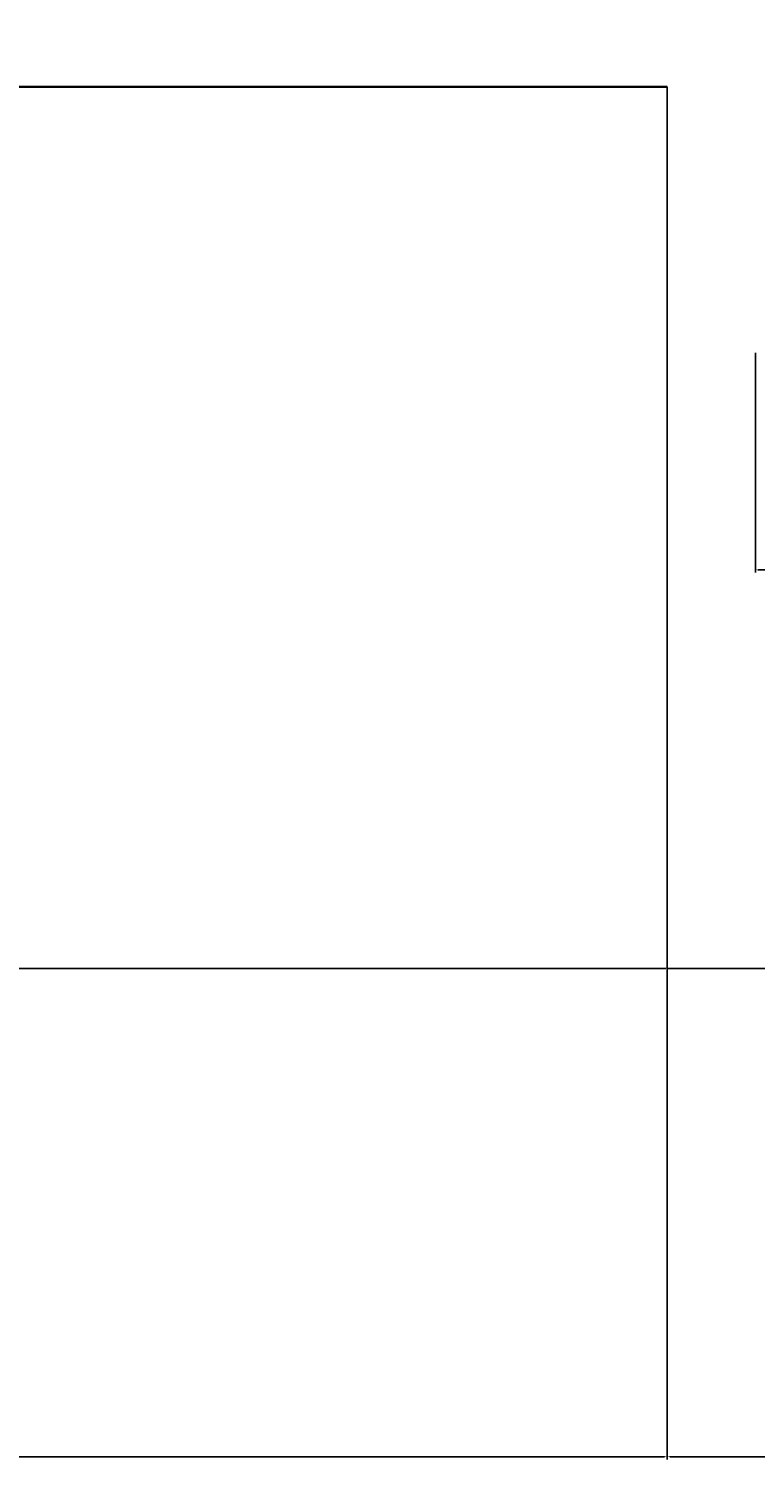
# Model space of a CAD drawing. Units: inches. Extents: x 4159 to 4826, y 299 to 1026.
# Tile 7 of 37: x 4404 to 4453, y 299 to 396. Entities that reach past the tile are written whole.
import ezdxf

# ---------------------------------------------------------------- set-up
doc = ezdxf.new("R2010")
doc.units = ezdxf.units.IN
for name, color, linetype, lineweight in [('A-ANNO-DIMS', 2, 'Continuous', 18), ('A-FLOR-STRS', 3, 'Continuous', 25), ('A-WALL', 7, 'Continuous', 35)]:
    doc.layers.add(name, color=color, linetype=linetype, lineweight=lineweight)
doc.styles.get("Standard").update_dxf_attribs({"font": 'arial.ttf'})
doc.dimstyles.get("Standard").update_dxf_attribs({"dimtxt": 0.18, "dimasz": 0.18, "dimexe": 0.18, "dimexo": 0.0625, "dimgap": 0.09, "dimtad": 0, "dimtih": 1, "dimtoh": 1, "dimdec": 4, "dimzin": 0, "dimdsep": 46, "dimtxsty": 'Standard', "dimcen": 0.09, "dimadec": 0, "dimazin": 0, "dimtfac": 1, "dimtdec": 4, "dimtofl": 0, "dimtmove": 0, "dimatfit": 3, "dimfxl": 1, "dimtolj": 1, "dimtzin": 0, "dimarcsym": 0})

# ---------------------------------------------------------------- blocks, each defined once
blk = doc.blocks.new('*D42')
at = {"layer": 'A-ANNO-DIMS', "color": 0, "lineweight": -2, "transparency": 16777216}
for p, q in [((4453.31, 374.133), (4453.31, 359.165)), ((4495.889, 374.133), (4495.889, 359.165)), ((4453.49, 359.345), (4474.068, 359.345)), ((4495.709, 359.345), (4475.131, 359.345))]:
    blk.add_line(p, q, dxfattribs=at)
at = {"layer": 'A-ANNO-DIMS', "color": 0, "transparency": 16777216}
for points in [[(4453.49, 359.375), (4453.49, 359.315), (4453.31, 359.345)], [(4495.709, 359.375), (4495.709, 359.315), (4495.889, 359.345)]]:
    blk.add_solid(points, dxfattribs=at)
at = {"layer": 'Defpoints', "color": 0, "transparency": 16777216}
for p in [(4453.31, 374.195), (4495.889, 374.195), (4495.889, 359.345)]:
    blk.add_point(p, dxfattribs=at)
at = {"layer": 'A-ANNO-DIMS', "color": 0, "transparency": 16777216, "insert": (4474.6, 359.345), "char_height": 0.18, "attachment_point": 5}
blk.add_mtext('\\A1;43 TYP.', dxfattribs=at)
blk = doc.blocks.new('*D44')
at = {"layer": 'A-ANNO-DIMS', "color": 0, "lineweight": -2, "transparency": 16777216}
for p, q in [((4287.263, 963.093), (4158.88, 963.093)), ((4159.06, 962.913), (4159.06, 647.826)), ((4159.06, 332.375), (4159.06, 647.462)), ((4447.248, 332.195), (4158.88, 332.195))]:
    blk.add_line(p, q, dxfattribs=at)
at = {"layer": 'A-ANNO-DIMS', "color": 0, "transparency": 16777216}
for points in [[(4159.03, 962.913), (4159.09, 962.913), (4159.06, 963.093)], [(4159.03, 332.375), (4159.09, 332.375), (4159.06, 332.195)]]:
    blk.add_solid(points, dxfattribs=at)
at = {"layer": 'Defpoints', "color": 0, "transparency": 16777216}
for p in [(4287.326, 963.093), (4159.06, 332.195), (4447.31, 332.195)]:
    blk.add_point(p, dxfattribs=at)
at = {"layer": 'A-ANNO-DIMS', "color": 0, "transparency": 16777216, "insert": (4159.06, 647.644), "char_height": 0.18, "attachment_point": 5}
blk.add_mtext('\\A1;630.9', dxfattribs=at)
blk = doc.blocks.new('*D46')
at = {"layer": 'A-ANNO-DIMS', "color": 0, "lineweight": -2, "transparency": 16777216}
for p, q in [((4192.31, 392.192), (4192.31, 298.765)), ((4447.31, 332.133), (4447.31, 298.765)), ((4192.49, 298.945), (4319.519, 298.945)), ((4447.13, 298.945), (4320.101, 298.945))]:
    blk.add_line(p, q, dxfattribs=at)
at = {"layer": 'A-ANNO-DIMS', "color": 0, "transparency": 16777216}
for points in [[(4192.49, 298.975), (4192.49, 298.915), (4192.31, 298.945)], [(4447.13, 298.975), (4447.13, 298.915), (4447.31, 298.945)]]:
    blk.add_solid(points, dxfattribs=at)
at = {"layer": 'Defpoints', "color": 0, "transparency": 16777216}
for p in [(4192.31, 392.254), (4447.31, 332.195), (4447.31, 298.945)]:
    blk.add_point(p, dxfattribs=at)
at = {"layer": 'A-ANNO-DIMS', "color": 0, "transparency": 16777216, "insert": (4319.81, 298.945), "char_height": 0.18, "attachment_point": 5}
blk.add_mtext('\\A1;255', dxfattribs=at)
blk = doc.blocks.new('*D47')
at = {"layer": 'A-ANNO-DIMS', "color": 0, "lineweight": -2, "transparency": 16777216}
for p, q in [((4447.31, 332.133), (4447.31, 298.765)), ((4547.889, 332.133), (4547.889, 298.765)), ((4447.49, 298.945), (4497.144, 298.945)), ((4547.709, 298.945), (4498.055, 298.945))]:
    blk.add_line(p, q, dxfattribs=at)
at = {"layer": 'A-ANNO-DIMS', "color": 0, "transparency": 16777216}
for points in [[(4447.49, 298.975), (4447.49, 298.915), (4447.31, 298.945)], [(4547.709, 298.975), (4547.709, 298.915), (4547.889, 298.945)]]:
    blk.add_solid(points, dxfattribs=at)
at = {"layer": 'Defpoints', "color": 0, "transparency": 16777216}
for p in [(4447.31, 332.195), (4547.889, 332.195), (4547.889, 298.945)]:
    blk.add_point(p, dxfattribs=at)
at = {"layer": 'A-ANNO-DIMS', "color": 0, "transparency": 16777216, "insert": (4497.6, 298.945), "char_height": 0.18, "attachment_point": 5}
blk.add_mtext('\\A1;100.58', dxfattribs=at)

msp = doc.modelspace()

# ---------------------------------------------------------------- linework, layer by layer
at = {"layer": 'A-FLOR-STRS'}
for p, q in [((4447.31, 392.254), (4447.31, 332.195)), ((4447.31, 332.195), (4547.889, 332.195))]:
    msp.add_line(p, q, dxfattribs=at)
at = {"layer": 'A-WALL'}
msp.add_line((4447.31, 392.254), (4369.31, 392.254), dxfattribs=at)

# ---------------------------------------------------------------- dimensions: what is measured, and where the dimension line sits
at = {"layer": 'A-ANNO-DIMS'}
dim = msp.add_linear_dim(base=(4159.06, 332.195), p1=(4287.326, 963.093), p2=(4447.31, 332.195), angle=90, dimstyle='Standard', override={"dimdec": 1, "dimlfac": 1, "dimrnd": 0, "dimzin": 0, "dimdsep": 46, "dimlunit": 2}, dxfattribs=at)
dim.commit()
dim.dimension.update_dxf_attribs({"geometry": '*D44', "text_midpoint": (4159.06, 647.644)})
for base, p1, p2, override, picture, middle in [((4447.31, 298.945), (4192.31, 392.254), (4447.31, 332.195), {"dimdec": 0, "dimlfac": 1, "dimrnd": 0, "dimzin": 0, "dimdsep": 46, "dimlunit": 2}, '*D46', (4319.81, 298.945)), ((4547.889, 298.945), (4447.31, 332.195), (4547.889, 332.195), {"dimdec": 2, "dimlfac": 1, "dimrnd": 0, "dimzin": 0, "dimdsep": 46, "dimlunit": 2}, '*D47', (4497.6, 298.945))]:
    dim = msp.add_linear_dim(base=base, p1=p1, p2=p2, dimstyle='Standard', override=override, dxfattribs=at)
    dim.commit()
    dim.dimension.update_dxf_attribs({"geometry": picture, "text_midpoint": middle})
dim = msp.add_linear_dim(base=(4495.889, 359.345), p1=(4453.31, 374.195), p2=(4495.889, 374.195), text='<> TYP.', dimstyle='Standard', override={"dimdec": 0, "dimlfac": 1, "dimrnd": 0, "dimzin": 0, "dimdsep": 46, "dimlunit": 2}, dxfattribs=at)
dim.commit()
dim.dimension.update_dxf_attribs({"geometry": '*D42', "text_midpoint": (4474.6, 359.345)})

doc.saveas('drawing.dxf')
